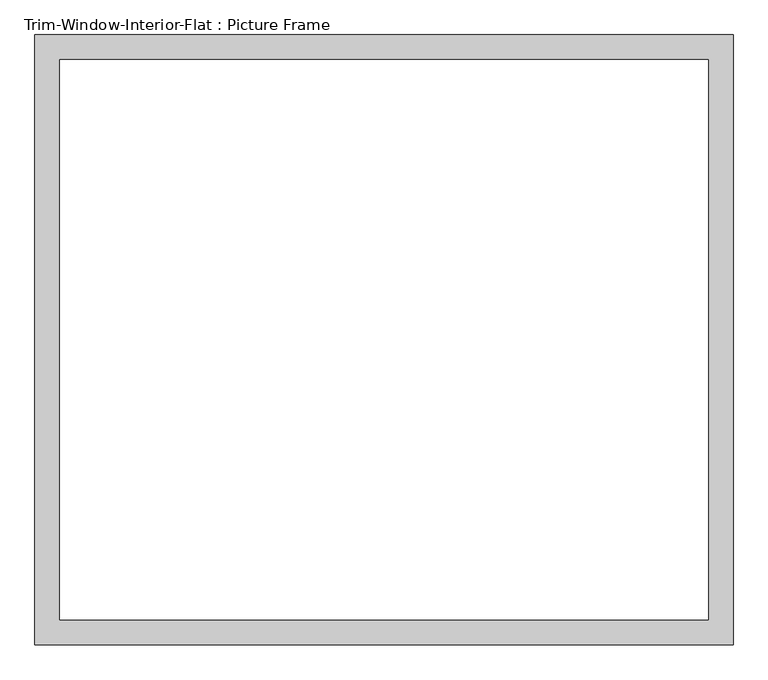
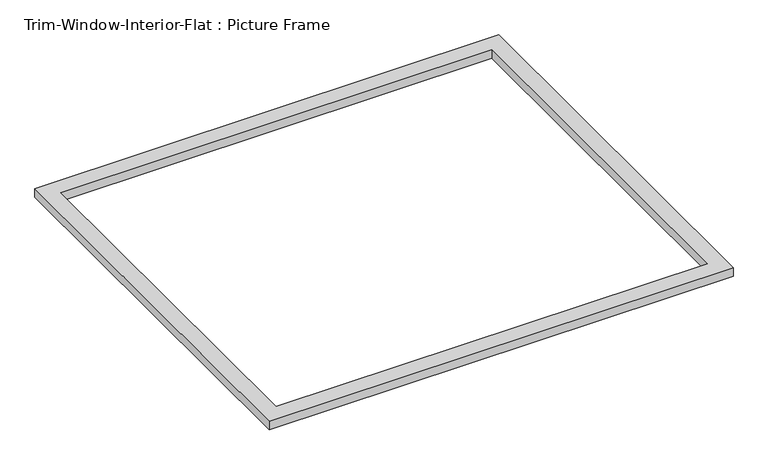
"""IFC4 building model written with IfcOpenShell, lengths in millimetres: proxy geometry, Trim-Window-Interior-Flat : Picture Frame."""

from ifc_helpers import new_model, si_unit, origin, origin_with_axes, place, context, project, spatial, polyline, outline, extrude, source, transform, mapped, element, save


def trim_window_interior_flat_picture_frame_e325e1d2(model_context):
    return source(origin(), model_context, "Body", "SweptSolid", [
        extrude(outline(polyline([(806.45, 44.45), (806.45, -1365.25), (-806.45, -1365.25), (-806.45, 44.45), (806.45, 44.45)]), holes=[polyline([(749.3, -12.7), (-749.3, -12.7), (-749.3, -1308.1), (749.3, -1308.1), (749.3, -12.7)])]), origin_with_axes(), (0.0, 0.0, 1.0), 31.75),
    ])


if __name__ == "__main__":
    model = new_model("IFC4")
    model_context = context("Model", 3, world=origin())
    ifc_project = project(units=[si_unit("LENGTHUNIT", "METRE", prefix="MILLI")], contexts=[model_context])
    site = spatial("IfcSite", under=ifc_project)
    building = spatial("IfcBuilding", under=site)
    placement = place(None, origin())
    trim_window_interior_flat_picture_frame_shape = trim_window_interior_flat_picture_frame_e325e1d2(model_context)
    element("IfcBuildingElementProxy", 1, Name="Trim-Window-Interior-Flat : Picture Frame", ObjectType="Trim-Window-Interior-Flat : Picture Frame", at=placement, inside=building, context=model_context, shape_type="MappedRepresentation", body=[
        mapped(trim_window_interior_flat_picture_frame_shape, transform((0.0, 0.0, 0.0), x_axis=(1.0, 0.0, 0.0), y_axis=(0.0, 1.0, 0.0), z_axis=(0.0, 0.0, 1.0))),
    ])
    save(model, "model.ifc")

# Revit data of these elements
# Type "Trim-Window-Interior-Flat : Picture Frame"
#   Trim Thickness_Picture Frame = 0' - 1 1/4"
#   Trim Width = 0' - 2 1/4"
#   Trim Thickness_with Sill = 0' - 0 3/4"
#   Sill Thickness = 0' - 1 1/4"
#   Opening Width [instance default] = 2' - 0"
#   Opening Height [instance default] = 3' - 0"
#   Default Elevation = 4' - 0"
#   Sill = no
#   Picture Frame = yes
#   Trim Material [instance default] = none
# Element 1 (IfcBuildingElementProxy, "Trim-Window-Interior-Flat : Picture Frame")
#   Opening Width = 5' - 0"
#   Opening Height = 4' - 4"
#   Trim Material = Wood - Stained
#   Materials on its faces: "Wood - Stained"
# Materials
#   "Wood - Stained": class "Wood", colour RGB 224 178 126, transparency 0, Cost = 0
